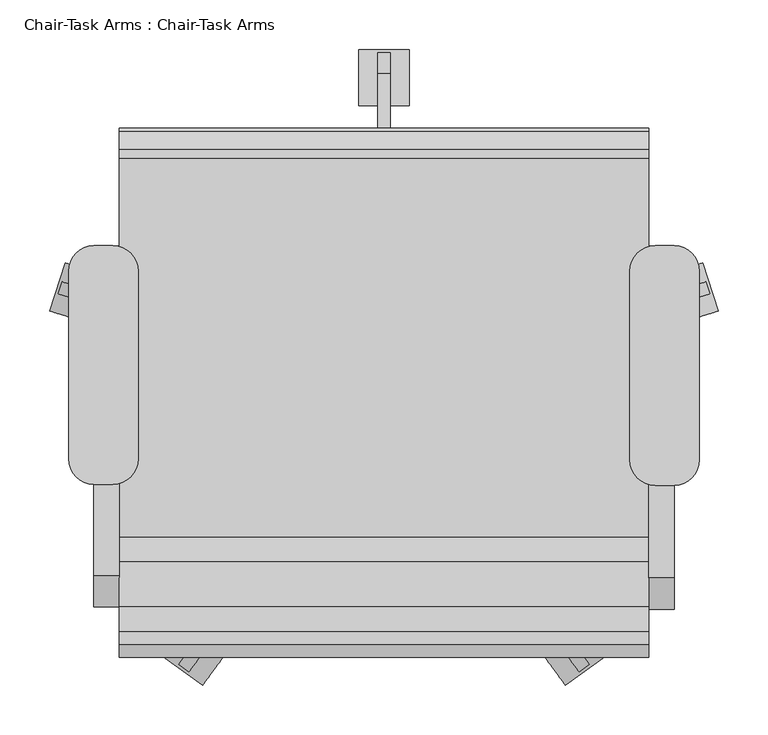
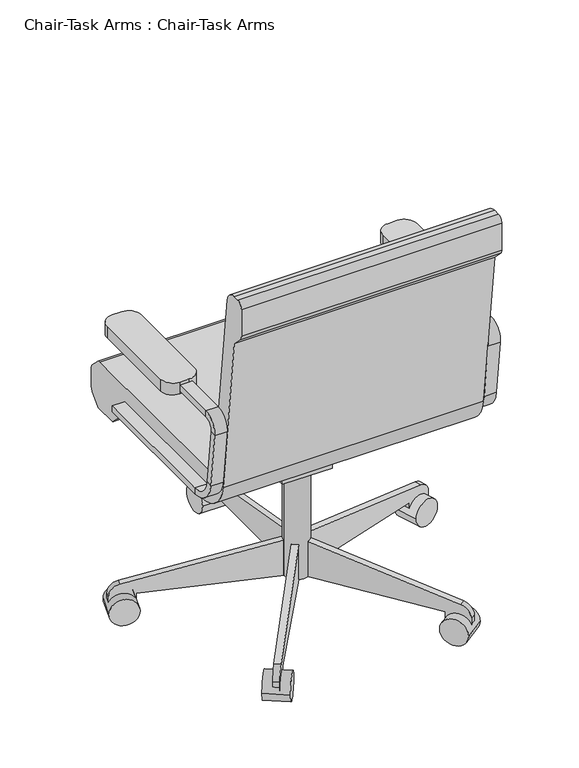
"""IFC4 building model written with IfcOpenShell, lengths in millimetres: furniture geometry, Chair-Task Arms : Chair-Task Arms."""

from ifc_helpers import new_model, si_unit, point, frame, frame_2d, origin, place, context, project, spatial, polyline, circle_curve, trimmed, segment, composite_curve, outline, extrude, source, transform, mapped, element, save
from ifc_brep_helpers import plane_surface, cylinder_surface, revolved_surface, advanced_brep


def chair_task_arms_chair_task_arms_fa5a08ef(model_context):
    return source(origin(), model_context, "Body", "SolidModel", [
        extrude(outline(composite_curve([segment(polyline([(433.0908197, -74.2028048), (414.0408197, -74.2028048)]), True, "CONTINUOUS"), segment(trimmed(circle_curve(frame_2d((414.0408197, -48.8028048)), 25.4), [point((414.0408197, -74.2028048))], [point((388.6408197, -48.8028048))], False, "CARTESIAN"), True, "CONTINUOUS"), segment(polyline([(388.6408197, -48.8028048), (388.6408197, 141.6319091)]), True, "CONTINUOUS"), segment(trimmed(circle_curve(frame_2d((414.0408197, 141.6319091)), 25.4), [point((388.6408197, 141.6319091))], [point((414.0408197, 167.0319091))], False, "CARTESIAN"), True, "CONTINUOUS"), segment(polyline([(414.0408197, 167.0319091), (433.0908197, 167.0319091)]), True, "CONTINUOUS"), segment(trimmed(circle_curve(frame_2d((433.0908197, 141.6319091)), 25.4), [point((433.0908197, 167.0319091))], [point((458.4908197, 141.6319091))], False, "CARTESIAN"), True, "CONTINUOUS"), segment(polyline([(458.4908197, 141.6319091), (458.4908197, -48.8028048)]), True, "CONTINUOUS"), segment(trimmed(circle_curve(frame_2d((433.0908197, -48.8028048)), 25.4), [point((458.4908197, -48.8028048))], [point((433.0908197, -74.2028048))], False, "CARTESIAN"), True, "CONTINUOUS")], self_intersect=False)), frame((0.0, 0.0, 596.9), z_axis=(0.0, 0.0, 1.0), x_axis=(1.0, 0.0, 0.0)), (0.0, 0.0, 1.0), 25.4),
        extrude(outline(composite_curve([segment(polyline([(-132.0591803, -73.1575984), (-151.1091803, -73.1575984)]), True, "CONTINUOUS"), segment(trimmed(circle_curve(frame_2d((-151.1091803, -47.7575984)), 25.4), [point((-151.1091803, -73.1575984))], [point((-176.5091803, -47.7575984))], False, "CARTESIAN"), True, "CONTINUOUS"), segment(polyline([(-176.5091803, -47.7575984), (-176.5091803, 141.6319091)]), True, "CONTINUOUS"), segment(trimmed(circle_curve(frame_2d((-151.1091803, 141.6319091)), 25.4), [point((-176.5091803, 141.6319091))], [point((-151.1091803, 167.0319091))], False, "CARTESIAN"), True, "CONTINUOUS"), segment(polyline([(-151.1091803, 167.0319091), (-132.0591803, 167.0319091)]), True, "CONTINUOUS"), segment(trimmed(circle_curve(frame_2d((-132.0591803, 141.6319091)), 25.4), [point((-132.0591803, 167.0319091))], [point((-106.6591803, 141.6319091))], False, "CARTESIAN"), True, "CONTINUOUS"), segment(polyline([(-106.6591803, 141.6319091), (-106.6591803, -47.7575984)]), True, "CONTINUOUS"), segment(trimmed(circle_curve(frame_2d((-132.0591803, -47.7575984)), 25.4), [point((-106.6591803, -47.7575984))], [point((-132.0591803, -73.1575984))], False, "CARTESIAN"), True, "CONTINUOUS")], self_intersect=False)), frame((0.0, 0.0, 596.9), z_axis=(0.0, 0.0, 1.0), x_axis=(1.0, 0.0, 0.0)), (0.0, 0.0, 1.0), 25.4),
        advanced_brep(
        [(-151.1091803, 167.0319091, 412.75), (-151.1091803, 167.0319091, 425.45), (-125.7091803, 167.0319091, 425.45), (-125.7091803, 167.0319091, 412.75), (-151.1091803, -126.2388651, 412.75), (-151.1091803, -126.2388651, 425.45), (-125.7091803, -126.2388651, 425.45), (-125.7091803, -126.2388651, 412.75), (-151.1091803, -170.3844094, 464.7064065), (-151.1091803, -182.9974221, 463.2225227), (-125.7091803, -170.3844094, 464.7064065), (-125.7091803, -182.9974221, 463.2225227), (-151.1091803, -196.7936301, 580.4902904), (-151.1091803, -184.1806174, 581.9741742), (-125.7091803, -184.1806174, 581.9741742), (-125.7091803, -196.7936301, 580.4902904), (-151.1091803, -165.2610984, 603.25), (-151.1091803, -165.2610984, 615.95), (-125.7091803, -165.2610984, 603.25), (-125.7091803, -165.2610984, 615.95), (-151.1091803, 18.9459016, 615.95), (-125.7091803, 18.9459016, 615.95), (-125.7091803, 18.9459016, 603.25), (-151.1091803, 18.9459016, 603.25)],
        [
            (0, 1),
            (1, 2),
            (2, 3),
            (3, 0),
            (0, 4),
            (4, 5),
            (5, 1),
            (5, 6),
            (6, 2),
            (6, 7),
            (7, 3),
            (7, 4),
            (8, 5, circle_curve(frame((-151.1091803, -126.2388651, 469.9), z_axis=(1.0, 0.0, 0.0), x_axis=(0.0, 0.0, -1.0)), 44.45)),
            (4, 9, circle_curve(frame((-151.1091803, -126.2388651, 469.9), z_axis=(-1.0, 0.0, 0.0), x_axis=(0.0, 0.0, -1.0)), 57.15)),
            (9, 8),
            (10, 6, circle_curve(frame((-125.7091803, -126.2388651, 469.9), z_axis=(1.0, 0.0, 0.0), x_axis=(0.0, 0.0, -1.0)), 44.45)),
            (8, 10),
            (11, 7, circle_curve(frame((-125.7091803, -126.2388651, 469.9), z_axis=(1.0, 0.0, 0.0), x_axis=(0.0, 0.0, -1.0)), 57.15)),
            (10, 11),
            (11, 9),
            (9, 12),
            (12, 13),
            (13, 8),
            (13, 14),
            (14, 10),
            (14, 15),
            (15, 11),
            (15, 12),
            (16, 13, circle_curve(frame((-151.1091803, -165.2610984, 584.2), z_axis=(1.0, 0.0, 0.0), x_axis=(0.0, -0.9931506043228768, -0.11684124756739202)), 19.05)),
            (12, 17, circle_curve(frame((-151.1091803, -165.2610984, 584.2), z_axis=(-1.0, 0.0, 0.0), x_axis=(0.0, -0.9931506043228768, -0.11684124756739202)), 31.75)),
            (17, 16),
            (18, 14, circle_curve(frame((-125.7091803, -165.2610984, 584.2), z_axis=(1.0, 0.0, 0.0), x_axis=(0.0, -0.9931506043228768, -0.11684124756739202)), 19.05)),
            (16, 18),
            (19, 15, circle_curve(frame((-125.7091803, -165.2610984, 584.2), z_axis=(1.0, 0.0, 0.0), x_axis=(0.0, -0.9931506043228768, -0.11684124756739202)), 31.75)),
            (18, 19),
            (19, 17),
            (20, 21),
            (21, 22),
            (22, 23),
            (23, 20),
            (17, 20),
            (23, 16),
            (22, 18),
            (21, 19),
        ],
        [
            plane_surface(frame((-152.608212, 167.0319091, 419.1), z_axis=(0.0, 1.0, 0.0), x_axis=(0.0, 0.0, -1.0))),
            plane_surface(frame((-151.1091803, 167.0319091, 412.75), z_axis=(-1.0, 0.0, 0.0), x_axis=(0.0, -1.0, 0.0))),
            plane_surface(frame((-151.1091803, 167.0319091, 425.45), z_axis=(0.0, 0.0, 1.0), x_axis=(0.0, -1.0, 0.0))),
            plane_surface(frame((-125.7091803, 167.0319091, 425.45), z_axis=(1.0, 0.0, 0.0), x_axis=(0.0, -1.0, 0.0))),
            plane_surface(frame((-125.7091803, 167.0319091, 412.75), z_axis=(0.0, 0.0, -1.0), x_axis=(0.0, -1.0, 0.0))),
            plane_surface(frame((-151.1091803, -126.2388651, 469.9), z_axis=(-1.0, 0.0, 0.0), x_axis=(0.0, 0.0, -1.0))),
            revolved_surface(polyline([(-151.1091803, -126.2388651, 425.45), (-125.7091803, -126.2388651, 425.45)]), (-138.4091803, -126.2388651, 469.9), (-1.0, 0.0, 0.0)),
            plane_surface(frame((-125.7091803, -126.2388651, 469.9), z_axis=(1.0, 0.0, 0.0), x_axis=(0.0, 0.0, -1.0))),
            cylinder_surface(frame((-138.4091803, -126.2388651, 469.9), z_axis=(-1.0, 0.0, 0.0), x_axis=(0.0, 0.0, -1.0)), 57.15),
            plane_surface(frame((-151.1091803, -182.9974221, 463.2225227), z_axis=(-1.0, 0.0, 0.0), x_axis=(0.0, -0.1168412475673856, 0.9931506043228776))),
            plane_surface(frame((-151.1091803, -170.3844094, 464.7064065), z_axis=(0.0, 0.9931506043228776, 0.1168412475673856), x_axis=(0.0, -0.1168412475673856, 0.9931506043228776))),
            plane_surface(frame((-125.7091803, -170.3844094, 464.7064065), z_axis=(1.0, 0.0, 0.0), x_axis=(0.0, -0.1168412475673856, 0.9931506043228776))),
            plane_surface(frame((-125.7091803, -182.9974221, 463.2225227), z_axis=(0.0, -0.9931506043228776, -0.1168412475673856), x_axis=(0.0, -0.1168412475673856, 0.9931506043228776))),
            plane_surface(frame((-151.1091803, -165.2610984, 584.2), z_axis=(-1.0, 0.0, 0.0), x_axis=(0.0, -0.9931506043228768, -0.11684124756739202))),
            revolved_surface(polyline([(-151.1091803, -184.1806174123508, 581.9741742338413), (-125.7091803, -184.1806174123508, 581.9741742338413)]), (-138.4091803, -165.2610984, 584.2), (-1.0, 0.0, 0.0)),
            plane_surface(frame((-125.7091803, -165.2610984, 584.2), z_axis=(1.0, 0.0, 0.0), x_axis=(0.0, -0.9931506043228768, -0.11684124756739202))),
            cylinder_surface(frame((-138.4091803, -165.2610984, 584.2), z_axis=(-1.0, 0.0, 0.0), x_axis=(0.0, -0.9931506043228768, -0.11684124756739202)), 31.75),
            plane_surface(frame((-152.608212, 18.9459016, 609.6), z_axis=(0.0, 1.0, 0.0), x_axis=(0.0, 0.0, 1.0))),
            plane_surface(frame((-151.1091803, -165.2610984, 615.95), z_axis=(-1.0, 0.0, 0.0), x_axis=(0.0, 1.0, 0.0))),
            plane_surface(frame((-151.1091803, -165.2610984, 603.25), z_axis=(0.0, 0.0, -1.0), x_axis=(0.0, 1.0, 0.0))),
            plane_surface(frame((-125.7091803, -165.2610984, 603.25), z_axis=(1.0, 0.0, 0.0), x_axis=(0.0, 1.0, 0.0))),
            plane_surface(frame((-125.7091803, -165.2610984, 615.95), z_axis=(0.0, 0.0, 1.0), x_axis=(0.0, 1.0, 0.0))),
        ],
        [
            (0, [[1, 2, 3, 4]]),
            (1, [[-1, 5, 6, 7]]),
            (2, [[-2, -7, 8, 9]]),
            (3, [[-3, -9, 10, 11]]),
            (4, [[-4, -11, 12, -5]]),
            (5, [[13, -6, 14, 15]]),
            (6, [[16, -8, -13, 17]]),
            (7, [[18, -10, -16, 19]]),
            (8, [[-14, -12, -18, 20]]),
            (9, [[-15, 21, 22, 23]]),
            (10, [[-17, -23, 24, 25]]),
            (11, [[-19, -25, 26, 27]]),
            (12, [[-20, -27, 28, -21]]),
            (13, [[29, -22, 30, 31]]),
            (14, [[32, -24, -29, 33]]),
            (15, [[34, -26, -32, 35]]),
            (16, [[-30, -28, -34, 36]]),
            (17, [[37, 38, 39, 40]]),
            (18, [[-31, 41, -40, 42]]),
            (19, [[-33, -42, -39, 43]]),
            (20, [[-35, -43, -38, 44]]),
            (21, [[-36, -44, -37, -41]]),
        ],
    ),
        advanced_brep(
        [(433.0908197, 167.0319091, 425.45), (433.0908197, 167.0319091, 412.75), (407.6908197, 167.0319091, 412.75), (407.6908197, 167.0319091, 425.45), (433.0908197, -128.329278, 425.45), (433.0908197, -128.329278, 412.75), (407.6908197, -128.329278, 412.75), (407.6908197, -128.329278, 425.45), (433.0908197, -185.0878351, 463.2225227), (433.0908197, -172.4748224, 464.7064065), (407.6908197, -185.0878351, 463.2225227), (407.6908197, -172.4748224, 464.7064065), (433.0908197, -186.2710303, 581.9741742), (433.0908197, -198.884043, 580.4902904), (407.6908197, -198.884043, 580.4902904), (407.6908197, -186.2710303, 581.9741742), (433.0908197, -167.3515113, 615.95), (433.0908197, -167.3515113, 603.25), (407.6908197, -167.3515113, 615.95), (407.6908197, -167.3515113, 603.25), (433.0908197, 18.9459016, 603.25), (407.6908197, 18.9459016, 603.25), (407.6908197, 18.9459016, 615.95), (433.0908197, 18.9459016, 615.95)],
        [
            (0, 1),
            (1, 2),
            (2, 3),
            (3, 0),
            (0, 4),
            (4, 5),
            (5, 1),
            (5, 6),
            (6, 2),
            (6, 7),
            (7, 3),
            (7, 4),
            (8, 5, circle_curve(frame((433.0908197, -128.329278, 469.9), z_axis=(1.0, 0.0, 0.0), x_axis=(0.0, 0.0, -1.0)), 57.15)),
            (4, 9, circle_curve(frame((433.0908197, -128.329278, 469.9), z_axis=(-1.0, 0.0, 0.0), x_axis=(0.0, 0.0, -1.0)), 44.45)),
            (9, 8),
            (10, 6, circle_curve(frame((407.6908197, -128.329278, 469.9), z_axis=(1.0, 0.0, 0.0), x_axis=(0.0, 0.0, -1.0)), 57.15)),
            (8, 10),
            (11, 7, circle_curve(frame((407.6908197, -128.329278, 469.9), z_axis=(1.0, 0.0, 0.0), x_axis=(0.0, 0.0, -1.0)), 44.45)),
            (10, 11),
            (11, 9),
            (9, 12),
            (12, 13),
            (13, 8),
            (13, 14),
            (14, 10),
            (14, 15),
            (15, 11),
            (15, 12),
            (16, 13, circle_curve(frame((433.0908197, -167.3515113, 584.2), z_axis=(1.0, 0.0, 0.0), x_axis=(0.0, -0.9931506043228767, -0.1168412475673929)), 31.75)),
            (12, 17, circle_curve(frame((433.0908197, -167.3515113, 584.2), z_axis=(-1.0, 0.0, 0.0), x_axis=(0.0, -0.9931506043228767, -0.1168412475673929)), 19.05)),
            (17, 16),
            (18, 14, circle_curve(frame((407.6908197, -167.3515113, 584.2), z_axis=(1.0, 0.0, 0.0), x_axis=(0.0, -0.9931506043228767, -0.1168412475673929)), 31.75)),
            (16, 18),
            (19, 15, circle_curve(frame((407.6908197, -167.3515113, 584.2), z_axis=(1.0, 0.0, 0.0), x_axis=(0.0, -0.9931506043228767, -0.1168412475673929)), 19.05)),
            (18, 19),
            (19, 17),
            (20, 21),
            (21, 22),
            (22, 23),
            (23, 20),
            (17, 20),
            (23, 16),
            (22, 18),
            (21, 19),
        ],
        [
            plane_surface(frame((406.191788, 167.0319091, 419.1), z_axis=(0.0, 1.0, 0.0), x_axis=(0.0, 0.0, -1.0))),
            plane_surface(frame((433.0908197, 167.0319091, 425.45), z_axis=(1.0, 0.0, 0.0), x_axis=(0.0, -1.0, 0.0))),
            plane_surface(frame((433.0908197, 167.0319091, 412.75), z_axis=(0.0, 0.0, -1.0), x_axis=(0.0, -1.0, 0.0))),
            plane_surface(frame((407.6908197, 167.0319091, 412.75), z_axis=(-1.0, 0.0, 0.0), x_axis=(0.0, -1.0, 0.0))),
            plane_surface(frame((407.6908197, 167.0319091, 425.45), z_axis=(0.0, 0.0, 1.0), x_axis=(0.0, -1.0, 0.0))),
            plane_surface(frame((433.0908197, -128.329278, 469.9), z_axis=(1.0, 0.0, 0.0), x_axis=(0.0, 0.0, -1.0))),
            cylinder_surface(frame((420.3908197, -128.329278, 469.9), z_axis=(-1.0, 0.0, 0.0), x_axis=(0.0, 0.0, -1.0)), 57.15),
            plane_surface(frame((407.6908197, -128.329278, 469.9), z_axis=(-1.0, 0.0, 0.0), x_axis=(0.0, 0.0, -1.0))),
            revolved_surface(polyline([(407.6908197, -128.329278, 425.45), (433.0908197, -128.329278, 425.45)]), (420.3908197, -128.329278, 469.9), (-1.0, 0.0, 0.0)),
            plane_surface(frame((433.0908197, -172.4748224, 464.7064065), z_axis=(1.0, 0.0, 0.0), x_axis=(0.0, -0.11684124756738626, 0.9931506043228775))),
            plane_surface(frame((433.0908197, -185.0878351, 463.2225227), z_axis=(0.0, -0.9931506043228775, -0.11684124756738655), x_axis=(0.0, -0.11684124756738655, 0.9931506043228775))),
            plane_surface(frame((407.6908197, -185.0878351, 463.2225227), z_axis=(-1.0, 0.0, 0.0), x_axis=(0.0, -0.11684124756738626, 0.9931506043228775))),
            plane_surface(frame((407.6908197, -172.4748224, 464.7064065), z_axis=(0.0, 0.9931506043228775, 0.11684124756738626), x_axis=(0.0, -0.11684124756738626, 0.9931506043228775))),
            plane_surface(frame((433.0908197, -167.3515113, 584.2), z_axis=(1.0, 0.0, 0.0), x_axis=(0.0, -0.9931506043228767, -0.1168412475673929))),
            cylinder_surface(frame((420.3908197, -167.3515113, 584.2), z_axis=(-1.0, 0.0, 0.0), x_axis=(0.0, -0.9931506043228767, -0.1168412475673929)), 31.75),
            plane_surface(frame((407.6908197, -167.3515113, 584.2), z_axis=(-1.0, 0.0, 0.0), x_axis=(0.0, -0.9931506043228767, -0.1168412475673929))),
            revolved_surface(polyline([(407.6908197, -186.2710303123508, 581.9741742338412), (433.0908197, -186.2710303123508, 581.9741742338412)]), (420.3908197, -167.3515113, 584.2), (-1.0, 0.0, 0.0)),
            plane_surface(frame((406.191788, 18.9459016, 609.6), z_axis=(0.0, 1.0, 0.0), x_axis=(0.0, 0.0, 1.0))),
            plane_surface(frame((433.0908197, -167.3515113, 603.25), z_axis=(1.0, 0.0, 0.0), x_axis=(0.0, 1.0, 0.0))),
            plane_surface(frame((433.0908197, -167.3515113, 615.95), z_axis=(0.0, 0.0, 1.0), x_axis=(0.0, 1.0, 0.0))),
            plane_surface(frame((407.6908197, -167.3515113, 615.95), z_axis=(-1.0, 0.0, 0.0), x_axis=(0.0, 1.0, 0.0))),
            plane_surface(frame((407.6908197, -167.3515113, 603.25), z_axis=(0.0, 0.0, -1.0), x_axis=(0.0, 1.0, 0.0))),
        ],
        [
            (0, [[1, 2, 3, 4]]),
            (1, [[-1, 5, 6, 7]]),
            (2, [[-2, -7, 8, 9]]),
            (3, [[-3, -9, 10, 11]]),
            (4, [[-4, -11, 12, -5]]),
            (5, [[13, -6, 14, 15]]),
            (6, [[16, -8, -13, 17]]),
            (7, [[18, -10, -16, 19]]),
            (8, [[-14, -12, -18, 20]]),
            (9, [[-15, 21, 22, 23]]),
            (10, [[-17, -23, 24, 25]]),
            (11, [[-19, -25, 26, 27]]),
            (12, [[-20, -27, 28, -21]]),
            (13, [[29, -22, 30, 31]]),
            (14, [[32, -24, -29, 33]]),
            (15, [[34, -26, -32, 35]]),
            (16, [[-30, -28, -34, 36]]),
            (17, [[37, 38, 39, 40]]),
            (18, [[-31, 41, -40, 42]]),
            (19, [[-33, -42, -39, 43]]),
            (20, [[-35, -43, -38, 44]]),
            (21, [[-36, -44, -37, -41]]),
        ],
    ),
        extrude(outline(composite_curve([segment(trimmed(circle_curve(frame_2d((140.9908197, 18.9459016)), 25.4), [point((115.5908197, 18.9459016))], [point((166.3908197, 18.9459016))], False, "CARTESIAN"), True, "CONTINUOUS"), segment(trimmed(circle_curve(frame_2d((140.9908197, 18.9459016)), 25.4), [point((166.3908197, 18.9459016))], [point((115.5908197, 18.9459016))], False, "CARTESIAN"), True, "CONTINUOUS")], self_intersect=False)), frame((0.0, 0.0, 53.5835944), z_axis=(0.0, 0.0, 1.0), x_axis=(1.0, 0.0, 0.0)), (0.0, 0.0, 1.0), 330.5914056),
        extrude(outline(composite_curve([segment(trimmed(circle_curve(frame_2d((0.0, -28.2002727)), 28.2002727), [point((0.0, -56.4005455))], [point((0.0, 0.0))], False, "CARTESIAN"), True, "CONTINUOUS"), segment(trimmed(circle_curve(frame_2d((0.0, -28.2002727)), 28.2002727), [point((0.0, 0.0))], [point((0.0, -56.4005455))], False, "CARTESIAN"), True, "CONTINUOUS")], self_intersect=False)), frame((477.6203484, 101.6163254, 28.1835944), z_axis=(-0.3090169943749423, 0.9510565162951553, 0.0), x_axis=(0.0, 0.0, 1.0)), (0.0, 0.0, 1.0), 50.8),
        extrude(outline(composite_curve([segment(polyline([(-25.4, 0.0), (0.0, 0.0), (0.0, -50.8), (-24.303053, -50.8)]), True, "CONTINUOUS"), segment(trimmed(circle_curve(frame_2d((-24.303053, -25.4)), 25.4), [point((-24.303053, -50.8))], [point((-49.3171699, -29.8106637))], False, "CARTESIAN"), True, "CONTINUOUS"), segment(polyline([(-49.3171699, -29.8106637), (-101.6, 266.7), (-101.6, 292.1), (-25.4, 292.1), (-25.4, 0.0)]), True, "CONTINUOUS")], self_intersect=False)), frame((420.756686, 103.1705568, 28.1835944), z_axis=(-0.3090169943749423, 0.9510565162951553, 0.0), x_axis=(0.0, 0.0, -1.0)), (0.0, 0.0, 1.0), 12.7),
        extrude(outline(composite_curve([segment(trimmed(circle_curve(frame_2d((0.0, -28.2002727)), 28.2002727), [point((0.0, -56.4005455))], [point((0.0, 0.0))], False, "CARTESIAN"), True, "CONTINUOUS"), segment(trimmed(circle_curve(frame_2d((0.0, -28.2002727)), 28.2002727), [point((0.0, 0.0))], [point((0.0, -56.4005455))], False, "CARTESIAN"), True, "CONTINUOUS")], self_intersect=False)), frame((323.63931, -275.6612394, 28.1835944), z_axis=(0.8090169943749499, 0.5877852522924699, 0.0), x_axis=(0.0, 0.0, 1.0)), (0.0, 0.0, 1.0), 50.8),
        extrude(outline(composite_curve([segment(polyline([(-25.4, 0.0), (0.0, 0.0), (0.0, -50.8), (-24.303053, -50.8)]), True, "CONTINUOUS"), segment(trimmed(circle_curve(frame_2d((-24.303053, -25.3999999)), 25.4), [point((-24.303053, -50.8))], [point((-49.3171699, -29.8106636))], False, "CARTESIAN"), True, "CONTINUOUS"), segment(polyline([(-49.3171699, -29.8106636), (-101.6, 266.7), (-101.6, 292.1), (-25.4, 292.1), (-25.4, 0.0)]), True, "CONTINUOUS")], self_intersect=False)), frame((307.545634, -221.1003988, 28.1835944), z_axis=(0.8090169943749499, 0.5877852522924699, 0.0), x_axis=(0.0, 0.0, -1.0)), (0.0, 0.0, 1.0), 12.7),
        extrude(outline(composite_curve([segment(trimmed(circle_curve(frame_2d((0.0, -28.2002727)), 28.2002727), [point((0.0, -56.4005455))], [point((0.0, 0.0))], False, "CARTESIAN"), True, "CONTINUOUS"), segment(trimmed(circle_curve(frame_2d((0.0, -28.2002727)), 28.2002727), [point((0.0, 0.0))], [point((0.0, -56.4005455))], False, "CARTESIAN"), True, "CONTINUOUS")], self_intersect=False)), frame((-41.6576707, -275.6612394, 28.1835944), z_axis=(-0.8090169943749458, 0.5877852522924754, 0.0), x_axis=(0.0, 0.0, -1.0)), (0.0, 0.0, 1.0), 50.8),
        extrude(outline(composite_curve([segment(polyline([(25.4, 0.0), (25.4, 292.1), (101.6, 292.1), (101.6, 266.7), (49.3171699, -29.8106637)]), True, "CONTINUOUS"), segment(trimmed(circle_curve(frame_2d((24.303053, -25.3999999)), 25.4), [point((49.3171699, -29.8106637))], [point((24.303053, -50.8))], False, "CARTESIAN"), True, "CONTINUOUS"), segment(polyline([(24.303053, -50.8), (0.0, -50.8), (0.0, 0.0), (25.4, 0.0)]), True, "CONTINUOUS")], self_intersect=False)), frame((-25.5639946, -221.1003988, 28.1835944), z_axis=(-0.8090169943749459, 0.5877852522924754, 0.0), x_axis=(0.0, 0.0, 1.0)), (0.0, 0.0, 1.0), 12.7),
        extrude(outline(composite_curve([segment(trimmed(circle_curve(frame_2d((0.0, -28.2002727)), 28.2002727), [point((0.0, -56.4005454))], [point((0.0, 0.0))], False, "CARTESIAN"), True, "CONTINUOUS"), segment(trimmed(circle_curve(frame_2d((0.0, -28.2002727)), 28.2002727), [point((0.0, 0.0))], [point((0.0, -56.4005454))], False, "CARTESIAN"), True, "CONTINUOUS")], self_intersect=False)), frame((-195.638709, 101.6163254, 28.1835944), z_axis=(0.3090169943749487, 0.9510565162951532, 0.0), x_axis=(0.0, 0.0, -1.0)), (0.0, 0.0, 1.0), 50.8),
        extrude(outline(composite_curve([segment(polyline([(25.4, 0.0), (25.4, 292.1000001), (101.6, 292.1000001), (101.6, 266.7), (49.3171699, -29.8106636)]), True, "CONTINUOUS"), segment(trimmed(circle_curve(frame_2d((24.303053, -25.4)), 25.4), [point((49.3171699, -29.8106636))], [point((24.303053, -50.8))], False, "CARTESIAN"), True, "CONTINUOUS"), segment(polyline([(24.303053, -50.8), (0.0, -50.8), (0.0, 0.0), (25.4, 0.0)]), True, "CONTINUOUS")], self_intersect=False)), frame((-138.7750467, 103.1705568, 28.1835944), z_axis=(0.3090169943749487, 0.9510565162951532, 0.0), x_axis=(0.0, 0.0, 1.0)), (0.0, 0.0, 1.0), 12.7),
        extrude(outline(composite_curve([segment(trimmed(circle_curve(frame_2d((336.4459016, 28.1835944)), 28.2002727), [point((308.2456289, 28.1835944))], [point((364.6461744, 28.1835944))], False, "CARTESIAN"), True, "CONTINUOUS"), segment(trimmed(circle_curve(frame_2d((336.4459016, 28.1835944)), 28.2002727), [point((364.6461744, 28.1835944))], [point((308.2456289, 28.1835944))], False, "CARTESIAN"), True, "CONTINUOUS")], self_intersect=False)), frame((115.5908197, 0.0, 0.0), z_axis=(1.0, 0.0, 0.0), x_axis=(0.0, 1.0, 0.0)), (0.0, 0.0, 1.0), 50.8),
        extrude(outline(composite_curve([segment(polyline([(311.0459016, 53.5835944), (18.9459016, 53.5835944), (18.9459016, 129.7835944), (44.3459016, 129.7835944), (340.8565654, 77.5007643)]), True, "CONTINUOUS"), segment(trimmed(circle_curve(frame_2d((336.4459016, 52.4866474)), 25.4), [point((340.8565654, 77.5007643))], [point((361.8459016, 52.4866474))], False, "CARTESIAN"), True, "CONTINUOUS"), segment(polyline([(361.8459016, 52.4866474), (361.8459016, 28.1835944), (311.0459016, 28.1835944), (311.0459016, 53.5835944)]), True, "CONTINUOUS")], self_intersect=False)), frame((134.6408197, 0.0, 0.0), z_axis=(1.0, 0.0, 0.0), x_axis=(0.0, 1.0, 0.0)), (0.0, 0.0, 1.0), 12.7),
        extrude(outline(polyline([(69.7459016, 383.7835944), (69.7459016, 371.0835944), (18.9459016, 283.0954134), (-19.1540984, 283.0954134), (-19.1540984, 383.7835944), (69.7459016, 383.7835944)])), frame((90.1908197, 0.0, 0.0), z_axis=(1.0, 0.0, 0.0), x_axis=(0.0, 1.0, 0.0)), (0.0, 0.0, 1.0), 101.6),
        extrude(outline(composite_curve([segment(polyline([(-126.2050455, 457.2), (255.0102301, 457.2)]), True, "CONTINUOUS"), segment(trimmed(circle_curve(frame_2d((255.0102301, 444.5)), 12.7), [point((255.0102301, 457.2))], [point((263.9604301, 453.510212))], False, "CARTESIAN"), True, "CONTINUOUS"), segment(polyline([(263.9604301, 453.510212), (281.8961016, 435.6939999)]), True, "CONTINUOUS"), segment(trimmed(circle_curve(frame_2d((272.9459016, 426.6837879)), 12.7), [point((281.8961016, 435.6939999))], [point((285.6459016, 426.6837879))], False, "CARTESIAN"), True, "CONTINUOUS"), segment(polyline([(285.6459016, 426.6837879), (285.6459016, 391.6405184)]), True, "CONTINUOUS"), segment(trimmed(circle_curve(frame_2d((260.2459016, 391.6405184)), 25.4), [point((285.6459016, 391.6405184))], [point((278.2663256, 373.7401184))], False, "CARTESIAN"), True, "CONTINUOUS"), segment(polyline([(278.2663256, 373.7401184), (260.2470284, 355.6), (209.4470284, 355.6), (181.0744602, 383.7835944), (-107.1089978, 383.7835944)]), True, "CONTINUOUS"), segment(trimmed(circle_curve(frame_2d((-107.1089978, 459.9835944)), 76.2), [point((-107.1089978, 383.7835944))], [point((-182.7870738, 451.0802913))], False, "CARTESIAN"), True, "CONTINUOUS"), segment(polyline([(-182.7870738, 451.0802913), (-222.3540984, 787.4), (-244.0343545, 809.0802561)]), True, "CONTINUOUS"), segment(trimmed(circle_curve(frame_2d((-235.0540984, 818.0605122)), 12.7), [point((-244.0343545, 809.0802561))], [point((-247.7540984, 818.0605122))], False, "CARTESIAN"), True, "CONTINUOUS"), segment(polyline([(-247.7540984, 818.0605122), (-247.7540984, 876.3)]), True, "CONTINUOUS"), segment(trimmed(circle_curve(frame_2d((-235.0540984, 876.3)), 12.7), [point((-247.7540984, 876.3))], [point((-235.0540984, 889.0))], False, "CARTESIAN"), True, "CONTINUOUS"), segment(polyline([(-235.0540984, 889.0), (-222.1789239, 889.0)]), True, "CONTINUOUS"), segment(trimmed(circle_curve(frame_2d((-222.1789239, 863.6)), 25.4), [point((-222.1789239, 889.0))], [point((-196.9528985, 866.5677677))], False, "CARTESIAN"), True, "CONTINUOUS"), segment(polyline([(-196.9528985, 866.5677677), (-151.4310708, 479.6322323)]), True, "CONTINUOUS"), segment(trimmed(circle_curve(frame_2d((-126.2050455, 482.6)), 25.4), [point((-151.4310708, 479.6322323))], [point((-126.2050455, 457.2))], True, "CARTESIAN"), True, "CONTINUOUS")], self_intersect=False)), frame((-125.7091803, 0.0, 0.0), z_axis=(1.0, 0.0, 0.0), x_axis=(0.0, 1.0, 0.0)), (0.0, 0.0, 1.0), 533.4),
    ])


if __name__ == "__main__":
    model = new_model("IFC4")
    model_context = context("Model", 3, world=origin())
    ifc_project = project(units=[si_unit("LENGTHUNIT", "METRE", prefix="MILLI")], contexts=[model_context])
    site = spatial("IfcSite", under=ifc_project)
    building = spatial("IfcBuilding", under=site)
    placement = place(None, origin())
    chair_task_arms_chair_task_arms_shape = chair_task_arms_chair_task_arms_fa5a08ef(model_context)
    element("IfcFurniture", 1, ObjectType="Chair-Task Arms : Chair-Task Arms", at=placement, inside=building, context=model_context, shape_type="MappedRepresentation", body=[
        mapped(chair_task_arms_chair_task_arms_shape, transform((0.0, 0.0, 0.0), x_axis=(1.0, 0.0, 0.0), y_axis=(0.0, 1.0, 0.0), z_axis=(0.0, 0.0, 1.0))),
    ])
    save(model, "model.ifc")

# Revit data of these elements
# Type "Chair-Task Arms : Chair-Task Arms"
#   Assembly Code = "E2020200"
#   Base Material = Plastic, Opaque Black
#   Caster Material = Plastic, Opaque Black
#   Seat/Back Material = Textile - Slate Blue
#   Default Elevation = 0
# Element 1 (IfcFurniture, "Chair-Task Arms : Chair-Task Arms")
#   Materials on its faces: "Plastic, Opaque Black", "Textile - Slate Blue"
# Materials
#   "Plastic, Opaque Black": class "Plastic", colour RGB 0 0 0, transparency 0.7, Description = "Plastic, generic, opaque black", Cost = 0
#   "Textile - Slate Blue": class "Fabric", colour RGB 98 102 118, transparency 0
